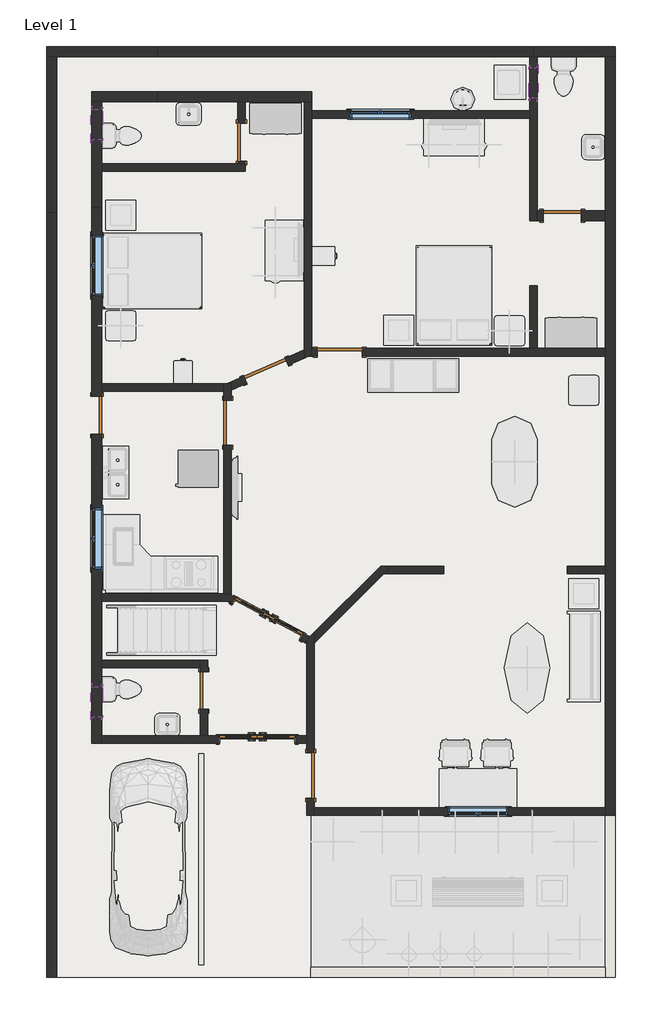
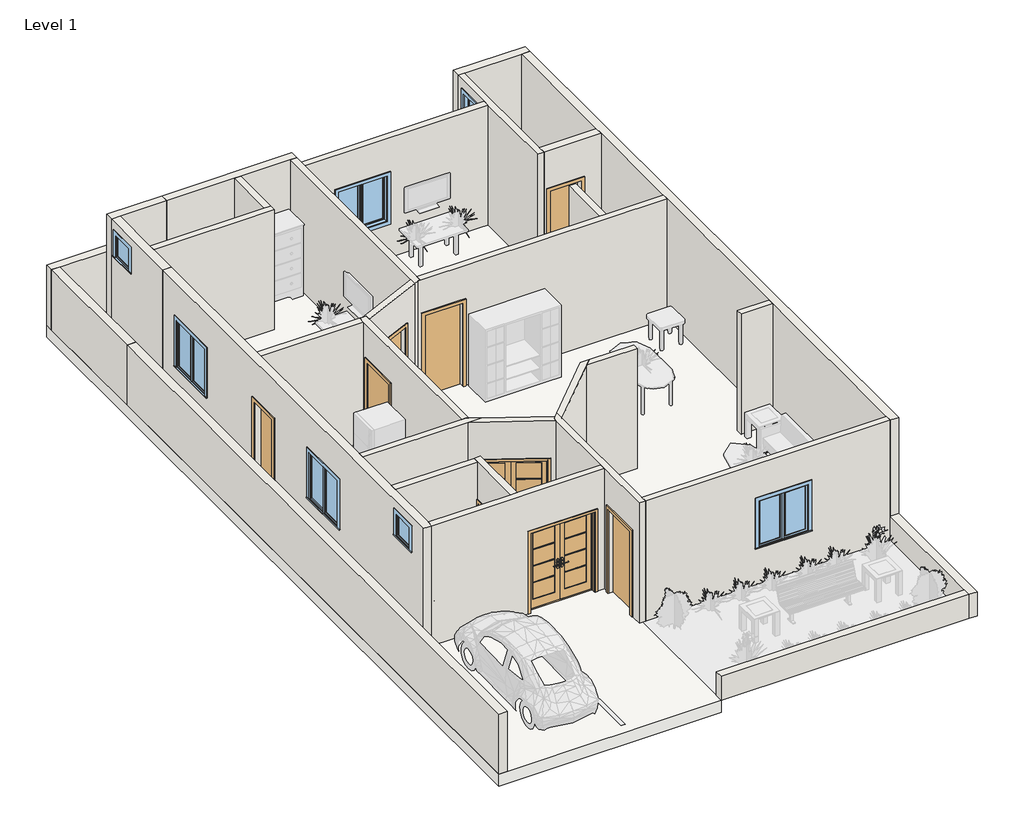
# One storey, part 1 of 2: 33 walls, 10 doors, 7 windows, 1 slab.
"""IFC4 building model written with IfcOpenShell, lengths in millimetres."""

from ifc_helpers import new_model, si_unit, frame, origin, origin_with_axes, place, context, project, spatial, polyline, outline, extrude, faceted_brep, transform, mapped, element, save
from components import door_94998e6c, door_255cab33, door_53b1b562, door_059fdd7e, door_16372e1c, door_686f89d2, window_0862ab64, window_be30da88, window_e41d21a6, window_3d781103

model = new_model("IFC4")

# Units and contexts
model_context = context("Model", 3, world=origin())
ifc_project = project(units=[si_unit("LENGTHUNIT", "METRE", prefix="MILLI")], contexts=[model_context])

# Site, building, storey
site = spatial("IfcSite", under=ifc_project)
building = spatial("IfcBuilding", under=site)
storey = spatial("IfcBuildingStorey", under=building, Name="Level 1", Elevation=0.0)

# Doors
placement = place(None, origin())
door_shape = door_94998e6c(model_context)
element("IfcDoor", 1, ObjectType="Door-Exterior-Double-Full Glass-Wood_Clad : 60\" x 80\"", at=placement, inside=storey, context=model_context, shape_type="MappedRepresentation", body=[
    mapped(door_shape, transform((-8581.0505662, -1172.4507293, 0.0), x_axis=(1.0, 0.0, 0.0), y_axis=(0.0, 1.0, 0.0), z_axis=(0.0, 0.0, 1.0))),
])
element("IfcDoor", 2, ObjectType="Door-Exterior-Double-Full Glass-Wood_Clad : 60\" x 80\"", at=placement, inside=storey, context=model_context, shape_type="MappedRepresentation", body=[
    mapped(door_shape, transform((-8368.5242285, 1268.0386954, 0.0), x_axis=(0.8838359385319597, -0.46779700058821444, 0.0), y_axis=(0.46779700058821444, 0.8838359385319597, 0.0), z_axis=(0.0, 0.0, 1.0))),
])
door_2_shape = door_255cab33(model_context)
element("IfcDoor", 3, ObjectType="Single-Flush : 30\" x 80\"", at=placement, inside=storey, context=model_context, shape_type="MappedRepresentation", body=[
    mapped(door_2_shape, transform((-8898.5505662, 10889.3742707, 0.0), x_axis=(0.0, -1.0, 0.0), y_axis=(1.0, 0.0, 0.0), z_axis=(0.0, 0.0, 1.0))),
])
door_3_shape = door_53b1b562(model_context)
element("IfcDoor", 4, ObjectType="Single-Flush : 30\" x 80\"", at=placement, inside=storey, context=model_context, shape_type="MappedRepresentation", body=[
    mapped(door_3_shape, transform((-11819.5505662, 5375.8598603, 0.0), x_axis=(0.0, 1.0, 0.0), y_axis=(-1.0, 0.0, 0.0), z_axis=(0.0, 0.0, 1.0))),
])
element("IfcDoor", 5, ObjectType="Single-Flush : 30\" x 80\"", at=placement, inside=storey, context=model_context, shape_type="MappedRepresentation", body=[
    mapped(door_3_shape, transform((-2421.5505662, 9403.5067625, 0.0), x_axis=(-1.0, 0.0, 0.0), y_axis=(0.0, -1.0, 0.0), z_axis=(0.0, 0.0, 1.0))),
])
door_4_shape = door_059fdd7e(model_context)
element("IfcDoor", 6, ObjectType="Single-Flush : 30\" x 80\"", at=placement, inside=storey, context=model_context, shape_type="MappedRepresentation", body=[
    mapped(door_4_shape, transform((-9660.5505662, -185.0257293, 0.0), x_axis=(0.0, 1.0, 0.0), y_axis=(-1.0, 0.0, 0.0), z_axis=(0.0, 0.0, 1.0))),
])
door_5_shape = door_16372e1c(model_context)
element("IfcDoor", 7, ObjectType="Single-Flush : 36\" x 84\"", at=placement, inside=storey, context=model_context, shape_type="MappedRepresentation", body=[
    mapped(door_5_shape, transform((-8406.3732014, 6273.0386879, 0.0), x_axis=(0.9158023090349923, 0.40162934500130426, 0.0), y_axis=(-0.40162934500130426, 0.9158023090349923, 0.0), z_axis=(0.0, 0.0, 1.0))),
])
element("IfcDoor", 8, ObjectType="Single-Flush : 36\" x 84\"", at=placement, inside=storey, context=model_context, shape_type="MappedRepresentation", body=[
    mapped(door_5_shape, transform((-9177.9505662, 5223.4598603, 0.0), x_axis=(0.0, 1.0, 0.0), y_axis=(-1.0, 0.0, 0.0), z_axis=(0.0, 0.0, 1.0))),
])
element("IfcDoor", 9, ObjectType="Single-Flush : 36\" x 84\"", at=placement, inside=storey, context=model_context, shape_type="MappedRepresentation", body=[
    mapped(door_5_shape, transform((-7501.5505662, -1899.5257293, 0.0), x_axis=(0.0, -1.0, 0.0), y_axis=(1.0, 0.0, 0.0), z_axis=(0.0, 0.0, 1.0))),
])
door_6_shape = door_686f89d2(model_context)
element("IfcDoor", 10, ObjectType="Single-Flush : 36\" x 84\"", at=placement, inside=storey, context=model_context, shape_type="MappedRepresentation", body=[
    mapped(door_6_shape, transform((-6917.3505662, 6647.5742707, 0.0), x_axis=(-1.0, 0.0, 0.0), y_axis=(0.0, -1.0, 0.0), z_axis=(0.0, 0.0, 1.0))),
])

# Slab
element("IfcSlab", 11, ObjectType="Generic - 12\"", at=placement, inside=storey, context=model_context, shape_type="SweptSolid", body=[
    extrude(outline(polyline([(-1354.7505662, 12819.7742707), (-1354.7505662, -2623.4257293), (-7501.5505662, -2623.4257293), (-7501.5505662, -5823.8257293), (-7501.5505662, -5976.2257293), (-12835.5505662, -5976.2257293), (-12835.5505662, 12819.7742707), (-1354.7505662, 12819.7742707)])), frame((0.0, 0.0, -304.8), z_axis=(0.0, 0.0, 1.0), x_axis=(1.0, 0.0, 0.0)), (0.0, 0.0, 1.0), 304.8),
])

# Walls
element("IfcWall", 12, ObjectType="Generic - 2'", at=placement, inside=storey, context=model_context, shape_type="SweptSolid", body=[
    extrude(outline(polyline([(-7501.5505662, -5773.0257293), (-1557.9505662, -5773.0257293), (-1557.9505662, -5976.2257293), (-7501.5505662, -5976.2257293), (-7501.5505662, -5773.0257293)])), origin_with_axes(), (0.0, 0.0, 1.0), 609.6),
])
element("IfcWall", 13, ObjectType="Generic - 2'", at=placement, inside=storey, context=model_context, shape_type="Brep", body=[
    faceted_brep([(-1557.9505662, -2623.4257293, 0.0), (-1557.9505662, -2699.6257293, 0.0), (-1557.9505662, -5773.0257293, 0.0), (-1557.9505662, -5976.2257293, 0.0), (-1557.9505662, -5976.2257293, 609.6), (-1557.9505662, -5773.0257293, 609.6), (-1557.9505662, -2623.4257293, 609.6), (-1354.7505662, -2623.4257293, 0.0), (-1354.7505662, -2623.4257293, 609.6), (-1354.7505662, -5976.2257293, 609.6), (-1354.7505662, -5976.2257293, 0.0)], [[[0, 1, 2, 3, 4, 5, 6]], [[7, 8, 9, 10]], [[3, 2, 1, 0, 7, 10]], [[6, 5, 4, 9, 8]], [[0, 6, 8, 7]], [[4, 3, 10, 9]]]),
])
element("IfcWall", 14, ObjectType="Generic - 8\"", at=placement, inside=storey, context=model_context, shape_type="Brep", body=[
    faceted_brep([(-1557.9505662, 12616.5742707, 0.0), (-1557.9505662, 9505.1067625, 0.0), (-1557.9505662, 9301.9067625, 0.0), (-1557.9505662, 6723.7742707, 0.0), (-1557.9505662, 6571.3742707, 0.0), (-1557.9505662, 2327.8598603, 0.0), (-1557.9505662, 2175.4598603, 0.0), (-1557.9505662, -2547.2257293, 0.0), (-1557.9505662, -2623.4257293, 0.0), (-1557.9505662, -2623.4257293, 609.6), (-1557.9505662, -2699.6257293, 609.6), (-1557.9505662, -2699.6257293, 3048.0), (-1557.9505662, -2547.2257293, 3048.0), (-1557.9505662, 2175.4598603, 3048.0), (-1557.9505662, 2327.8598603, 3048.0), (-1557.9505662, 6571.3742707, 3048.0), (-1557.9505662, 6723.7742707, 3048.0), (-1557.9505662, 9301.9067625, 3048.0), (-1557.9505662, 9505.1067625, 3048.0), (-1557.9505662, 12616.5742707, 3048.0), (-1354.7505662, 12616.5742707, 0.0), (-1354.7505662, 12616.5742707, 3048.0), (-1354.7505662, -2699.6257293, 3048.0), (-1354.7505662, -2699.6257293, 609.6), (-1354.7505662, -2623.4257293, 609.6), (-1354.7505662, -2623.4257293, 0.0)], [[[0, 1, 2, 3, 4, 5, 6, 7, 8, 9, 10, 11, 12, 13, 14, 15, 16, 17, 18, 19]], [[20, 21, 22, 23, 24, 25]], [[8, 7, 6, 5, 4, 3, 2, 1, 0, 20, 25]], [[0, 19, 21, 20]], [[9, 8, 25, 24]], [[23, 10, 9, 24]], [[11, 10, 23, 22]], [[19, 18, 17, 16, 15, 14, 13, 12, 11, 22, 21]]]),
])
element("IfcWall", 15, ObjectType="Generic - 8\"", at=placement, inside=storey, context=model_context, shape_type="Brep", body=[
    faceted_brep([(-7476.1505662, 11905.3742707, 0.0), (-10600.3505662, 11905.3742707, 0.0), (-10600.3505662, 11905.3742707, 3048.0), (-7476.1505662, 11905.3742707, 3048.0), (-7476.1505662, 11702.1742707, 0.0), (-7476.1505662, 11702.1742707, 3048.0), (-7628.5505662, 11702.1742707, 3048.0), (-8822.3505662, 11702.1742707, 3048.0), (-8974.7505662, 11702.1742707, 3048.0), (-10600.3505662, 11702.1742707, 3048.0), (-10600.3505662, 11702.1742707, 0.0), (-8974.7505662, 11702.1742707, 0.0), (-8822.3505662, 11702.1742707, 0.0), (-7628.5505662, 11702.1742707, 0.0)], [[[0, 1, 2, 3]], [[4, 5, 6, 7, 8, 9, 10, 11, 12, 13]], [[1, 0, 4, 13, 12, 11, 10]], [[2, 1, 10, 9]], [[0, 3, 5, 4]], [[3, 2, 9, 8, 7, 6, 5]]]),
])
element("IfcWall", 16, ObjectType="Generic - 8\"", at=placement, inside=storey, context=model_context, shape_type="Brep", body=[
    faceted_brep([(-11717.9505662, 5756.8598603, 2032.0), (-11717.9505662, 5756.8598603, 0.0), (-11717.9505662, 5858.4598603, 0.0), (-11717.9505662, 6010.8598603, 0.0), (-11717.9505662, 9568.5742707, 0.0), (-11717.9505662, 9568.5742707, 3048.0), (-11717.9505662, 6010.8598603, 3048.0), (-11717.9505662, 5858.4598603, 3048.0), (-11717.9505662, 1769.0598603, 3048.0), (-11717.9505662, 1616.6598603, 3048.0), (-11717.9505662, 424.5742707, 3048.0), (-11717.9505662, 272.1742707, 3048.0), (-11717.9505662, -1099.4257293, 3048.0), (-11717.9505662, -1251.8257293, 3048.0), (-11717.9505662, -1251.8257293, 0.0), (-11717.9505662, -1099.4257293, 0.0), (-11717.9505662, 272.1742707, 0.0), (-11717.9505662, 424.5742707, 0.0), (-11717.9505662, 1616.6598603, 0.0), (-11717.9505662, 1769.0598603, 0.0), (-11717.9505662, 4994.8598603, 0.0), (-11717.9505662, 4994.8598603, 2032.0), (-11717.9505662, 9009.7742707, 2133.6), (-11717.9505662, 9009.7742707, 914.4), (-11717.9505662, 7790.5742707, 914.4), (-11717.9505662, 7790.5742707, 2133.6), (-11717.9505662, 3496.2598603, 2133.6), (-11717.9505662, 3496.2598603, 914.4), (-11717.9505662, 2277.0598603, 914.4), (-11717.9505662, 2277.0598603, 2133.6), (-11717.9505662, -108.8257293, 2768.6), (-11717.9505662, -108.8257293, 2159.0), (-11717.9505662, -718.4257293, 2159.0), (-11717.9505662, -718.4257293, 2768.6), (-11921.1505662, 9568.5742707, 0.0), (-11921.1505662, 5756.8598603, 0.0), (-11921.1505662, 5756.8598603, 2032.0), (-11921.1505662, 4994.8598603, 2032.0), (-11921.1505662, 4994.8598603, 0.0), (-11921.1505662, -1251.8257293, 0.0), (-11921.1505662, -1251.8257293, 3048.0), (-11921.1505662, 9568.5742707, 3048.0), (-11921.1505662, 9009.7742707, 2133.6), (-11921.1505662, 7790.5742707, 2133.6), (-11921.1505662, 7790.5742707, 914.4), (-11921.1505662, 9009.7742707, 914.4), (-11921.1505662, 3496.2598603, 2133.6), (-11921.1505662, 2277.0598603, 2133.6), (-11921.1505662, 2277.0598603, 914.4), (-11921.1505662, 3496.2598603, 914.4), (-11921.1505662, -108.8257293, 2768.6), (-11921.1505662, -718.4257293, 2768.6), (-11921.1505662, -718.4257293, 2159.0), (-11921.1505662, -108.8257293, 2159.0)], [[[0, 1, 2, 3, 4, 5, 6, 7, 8, 9, 10, 11, 12, 13, 14, 15, 16, 17, 18, 19, 20, 21], [22, 23, 24, 25], [26, 27, 28, 29], [30, 31, 32, 33]], [[34, 35, 36, 37, 38, 39, 40, 41], [42, 43, 44, 45], [46, 47, 48, 49], [50, 51, 52, 53]], [[20, 19, 18, 17, 16, 15, 14, 39, 38]], [[4, 3, 2, 1, 35, 34]], [[5, 4, 34, 41]], [[14, 13, 40, 39]], [[36, 35, 1, 0]], [[37, 36, 0, 21]], [[38, 37, 21, 20]], [[23, 22, 42, 45]], [[24, 23, 45, 44]], [[25, 24, 44, 43]], [[22, 25, 43, 42]], [[27, 26, 46, 49]], [[28, 27, 49, 48]], [[29, 28, 48, 47]], [[26, 29, 47, 46]], [[31, 30, 50, 53]], [[32, 31, 53, 52]], [[33, 32, 52, 51]], [[30, 33, 51, 50]], [[13, 12, 11, 10, 9, 8, 7, 6, 5, 41, 40]]]),
])
element("IfcWall", 17, ObjectType="Generic - 8\"", at=placement, inside=storey, context=model_context, shape_type="Brep", body=[
    faceted_brep([(-10600.3505662, 11905.3742707, 0.0), (-11921.1505662, 11905.3742707, 0.0), (-11921.1505662, 11905.3742707, 3048.0), (-10600.3505662, 11905.3742707, 3048.0), (-10600.3505662, 11702.1742707, 0.0), (-10600.3505662, 11702.1742707, 3048.0), (-11717.9505662, 11702.1742707, 3048.0), (-11921.1505662, 11702.1742707, 3048.0), (-11921.1505662, 11702.1742707, 0.0), (-11717.9505662, 11702.1742707, 0.0)], [[[0, 1, 2, 3]], [[4, 5, 6, 7, 8, 9]], [[1, 0, 4, 9, 8]], [[0, 3, 5, 4]], [[2, 1, 8, 7]], [[3, 2, 7, 6, 5]]]),
])
element("IfcWall", 18, ObjectType="Generic - 8\"", at=placement, inside=storey, context=model_context, shape_type="Brep", body=[
    faceted_brep([(-11717.9505662, 9568.5742707, 0.0), (-11717.9505662, 10305.1742707, 0.0), (-11717.9505662, 10457.5742707, 0.0), (-11717.9505662, 11702.1742707, 0.0), (-11717.9505662, 11702.1742707, 3048.0), (-11717.9505662, 10457.5742707, 3048.0), (-11717.9505662, 10305.1742707, 3048.0), (-11717.9505662, 9568.5742707, 3048.0), (-11717.9505662, 11549.7742707, 2768.6), (-11717.9505662, 11549.7742707, 2159.0), (-11717.9505662, 10940.1742707, 2159.0), (-11717.9505662, 10940.1742707, 2768.6), (-11921.1505662, 9568.5742707, 0.0), (-11921.1505662, 9568.5742707, 3048.0), (-11921.1505662, 11702.1742707, 3048.0), (-11921.1505662, 11702.1742707, 0.0), (-11921.1505662, 11549.7742707, 2768.6), (-11921.1505662, 10940.1742707, 2768.6), (-11921.1505662, 10940.1742707, 2159.0), (-11921.1505662, 11549.7742707, 2159.0)], [[[0, 1, 2, 3, 4, 5, 6, 7], [8, 9, 10, 11]], [[12, 13, 14, 15], [16, 17, 18, 19]], [[3, 2, 1, 0, 12, 15]], [[0, 7, 13, 12]], [[4, 3, 15, 14]], [[9, 8, 16, 19]], [[10, 9, 19, 18]], [[11, 10, 18, 17]], [[8, 11, 17, 16]], [[7, 6, 5, 4, 14, 13]]]),
])
element("IfcWall", 19, ObjectType="Generic - 8\"", at=placement, inside=storey, context=model_context, shape_type="SweptSolid", body=[
    extrude(outline(polyline([(0.0, -2929.5505662), (0.0, -2802.5505662), (2032.0, -2802.5505662), (2032.0, -2040.5505662), (0.0, -2040.5505662), (0.0, -1557.9505662), (3048.0, -1557.9505662), (3048.0, -2929.5505662), (0.0, -2929.5505662)])), frame((0.0, 9301.9067625, 0.0), z_axis=(0.0, 1.0, 0.0), x_axis=(0.0, 0.0, 1.0)), (0.0, 0.0, 1.0), 203.2),
])
element("IfcWall", 20, ObjectType="Generic - 8\"", at=placement, inside=storey, context=model_context, shape_type="Brep", body=[
    faceted_brep([(-3005.7505662, 12616.5742707, 0.0), (-2929.5505662, 12616.5742707, 0.0), (-1557.9505662, 12616.5742707, 0.0), (-1354.7505662, 12616.5742707, 0.0), (-1354.7505662, 12616.5742707, 3048.0), (-1557.9505662, 12616.5742707, 3048.0), (-2929.5505662, 12616.5742707, 3048.0), (-3081.9505662, 12616.5742707, 3048.0), (-3081.9505662, 12616.5742707, 1524.0), (-3005.7505662, 12616.5742707, 1524.0), (-3005.7505662, 12819.7742707, 0.0), (-3005.7505662, 12819.7742707, 1524.0), (-3081.9505662, 12819.7742707, 1524.0), (-3081.9505662, 12819.7742707, 3048.0), (-1354.7505662, 12819.7742707, 3048.0), (-1354.7505662, 12819.7742707, 0.0)], [[[0, 1, 2, 3, 4, 5, 6, 7, 8, 9]], [[10, 11, 12, 13, 14, 15]], [[3, 2, 1, 0, 10, 15]], [[4, 3, 15, 14]], [[0, 9, 11, 10]], [[8, 12, 11, 9]], [[8, 7, 13, 12]], [[7, 6, 5, 4, 14, 13]]]),
])
element("IfcWall", 21, ObjectType="INNER 6\"", at=placement, inside=storey, context=model_context, shape_type="Brep", body=[
    faceted_brep([(-7628.5505662, 11702.1742707, 0.0), (-7628.5505662, 6697.3621381, 0.0), (-7628.5505662, 6530.9506774, 0.0), (-7628.5505662, 6530.9506774, 3048.0), (-7628.5505662, 6697.3621381, 3048.0), (-7628.5505662, 11702.1742707, 3048.0), (-7476.1505662, 11702.1742707, 0.0), (-7476.1505662, 11702.1742707, 3048.0), (-7476.1505662, 11524.3742707, 3048.0), (-7476.1505662, 11371.9742707, 3048.0), (-7476.1505662, 6723.7742707, 3048.0), (-7476.1505662, 6597.7864034, 3048.0), (-7476.1505662, 6597.7864034, 0.0), (-7476.1505662, 6723.7742707, 0.0), (-7476.1505662, 11371.9742707, 0.0), (-7476.1505662, 11524.3742707, 0.0), (-7536.3759763, 6571.3742707, 0.0), (-7536.3759763, 6571.3742707, 3048.0)], [[[0, 1, 2, 3, 4, 5]], [[6, 7, 8, 9, 10, 11, 12, 13, 14, 15]], [[2, 1, 0, 6, 15, 14, 13, 12, 16]], [[0, 5, 7, 6]], [[3, 2, 16, 12, 11, 17]], [[5, 4, 3, 17, 11, 10, 9, 8, 7]]]),
])
element("IfcWall", 22, ObjectType="INNER 6\"", at=placement, inside=storey, context=model_context, shape_type="Brep", body=[
    faceted_brep([(-7577.7505662, -2356.7257293, 2133.6), (-7577.7505662, -2356.7257293, 0.0), (-7577.7505662, -2699.6257293, 0.0), (-7577.7505662, -2699.6257293, 3048.0), (-7577.7505662, -1251.8257293, 3048.0), (-7577.7505662, -1099.4257293, 3048.0), (-7577.7505662, 759.6903382, 3048.0), (-7577.7505662, 837.1373442, 3048.0), (-7577.7505662, 837.1373442, 0.0), (-7577.7505662, 759.6903382, 0.0), (-7577.7505662, -1099.4257293, 0.0), (-7577.7505662, -1251.8257293, 0.0), (-7577.7505662, -1442.3257293, 0.0), (-7577.7505662, -1442.3257293, 2133.6), (-7425.3505662, -2699.6257293, 0.0), (-7425.3505662, -2547.2257293, 0.0), (-7425.3505662, -2356.7257293, 0.0), (-7425.3505662, -2356.7257293, 2133.6), (-7425.3505662, -1442.3257293, 2133.6), (-7425.3505662, -1442.3257293, 0.0), (-7425.3505662, 774.0111973, 0.0), (-7425.3505662, 989.5373442, 0.0), (-7425.3505662, 989.5373442, 3048.0), (-7425.3505662, 774.0111973, 3048.0), (-7425.3505662, -2547.2257293, 3048.0), (-7425.3505662, -2699.6257293, 3048.0), (-7515.6408392, 899.2470712, 0.0), (-7515.6408392, 899.2470712, 3048.0)], [[[0, 1, 2, 3, 4, 5, 6, 7, 8, 9, 10, 11, 12, 13]], [[14, 15, 16, 17, 18, 19, 20, 21, 22, 23, 24, 25]], [[2, 1, 16, 15, 14]], [[12, 11, 10, 9, 8, 26, 21, 20, 19]], [[3, 2, 14, 25]], [[8, 7, 27, 22, 21, 26]], [[17, 16, 1, 0]], [[18, 17, 0, 13]], [[19, 18, 13, 12]], [[7, 6, 5, 4, 3, 25, 24, 23, 22, 27]]]),
])
element("IfcWall", 23, ObjectType="INNER 6\"", at=placement, inside=storey, context=model_context, shape_type="Brep", body=[
    faceted_brep([(-7425.3505662, -2699.6257293, 0.0), (-1557.9505662, -2699.6257293, 0.0), (-1557.9505662, -2699.6257293, 609.6), (-1557.9505662, -2699.6257293, 3048.0), (-7425.3505662, -2699.6257293, 3048.0), (-4732.9505662, -2699.6257293, 2133.6), (-3513.7505662, -2699.6257293, 2133.6), (-3513.7505662, -2699.6257293, 914.4), (-4732.9505662, -2699.6257293, 914.4), (-7425.3505662, -2547.2257293, 0.0), (-7425.3505662, -2547.2257293, 3048.0), (-1557.9505662, -2547.2257293, 3048.0), (-1557.9505662, -2547.2257293, 0.0), (-4732.9505662, -2547.2257293, 2133.6), (-4732.9505662, -2547.2257293, 914.4), (-3513.7505662, -2547.2257293, 914.4), (-3513.7505662, -2547.2257293, 2133.6), (-1557.9505662, -2623.4257293, 0.0)], [[[0, 1, 2, 3, 4], [5, 6, 7, 8]], [[9, 10, 11, 12], [13, 14, 15, 16]], [[1, 0, 9, 12, 17]], [[0, 4, 10, 9]], [[14, 13, 5, 8]], [[15, 14, 8, 7]], [[16, 15, 7, 6]], [[13, 16, 6, 5]], [[1, 17, 12, 11, 3, 2]], [[4, 3, 11, 10]]]),
])
element("IfcWall", 24, ObjectType="INNER 6\"", at=placement, inside=storey, context=model_context, shape_type="Brep", body=[
    faceted_brep([(-7577.7505662, -1099.4257293, 3048.0), (-7577.7505662, -1099.4257293, 0.0), (-7793.6505662, -1099.4257293, 0.0), (-7793.6505662, -1099.4257293, 2057.4), (-9368.4505662, -1099.4257293, 2057.4), (-9368.4505662, -1099.4257293, 0.0), (-9584.3505662, -1099.4257293, 0.0), (-9736.7505662, -1099.4257293, 0.0), (-11717.9505662, -1099.4257293, 0.0), (-11717.9505662, -1099.4257293, 3048.0), (-9736.7505662, -1099.4257293, 3048.0), (-9584.3505662, -1099.4257293, 3048.0), (-7577.7505662, -1251.8257293, 0.0), (-7577.7505662, -1251.8257293, 3048.0), (-11717.9505662, -1251.8257293, 3048.0), (-11717.9505662, -1251.8257293, 0.0), (-9368.4505662, -1251.8257293, 0.0), (-9368.4505662, -1251.8257293, 2057.4), (-7793.6505662, -1251.8257293, 2057.4), (-7793.6505662, -1251.8257293, 0.0)], [[[0, 1, 2, 3, 4, 5, 6, 7, 8, 9, 10, 11]], [[12, 13, 14, 15, 16, 17, 18, 19]], [[1, 12, 19, 2]], [[15, 8, 7, 6, 5, 16]], [[1, 0, 13, 12]], [[9, 8, 15, 14]], [[18, 3, 2, 19]], [[3, 18, 17, 4]], [[4, 17, 16, 5]], [[0, 11, 10, 9, 14, 13]]]),
])
element("IfcWall", 25, ObjectType="INNER 6\"", at=placement, inside=storey, context=model_context, shape_type="Brep", body=[
    faceted_brep([(-7425.3505662, 774.0111973, 0.0), (-6023.9019032, 2175.4598603, 0.0), (-5871.5019032, 2327.8598603, 0.0), (-5871.5019032, 2327.8598603, 3048.0), (-6023.9019032, 2175.4598603, 3048.0), (-7425.3505662, 774.0111973, 3048.0), (-7425.3505662, 989.5373442, 0.0), (-7425.3505662, 989.5373442, 3048.0), (-6087.0280501, 2327.8598603, 3048.0), (-6087.0280501, 2327.8598603, 0.0)], [[[0, 1, 2, 3, 4, 5]], [[6, 7, 8, 9]], [[2, 1, 0, 6, 9]], [[0, 5, 7, 6]], [[3, 2, 9, 8]], [[5, 4, 3, 8, 7]]]),
])
element("IfcWall", 26, ObjectType="INNER 6\"", at=placement, inside=storey, context=model_context, shape_type="SweptSolid", body=[
    extrude(outline(polyline([(-4810.8649766, 2175.4598603), (-6023.9019032, 2175.4598603), (-5871.5019032, 2327.8598603), (-4810.8649766, 2327.8598603), (-4810.8649766, 2175.4598603)])), origin_with_axes(), (0.0, 0.0, 1.0), 3048.0),
])
element("IfcWall", 27, ObjectType="INNER 6\"", at=placement, inside=storey, context=model_context, shape_type="Brep", body=[
    faceted_brep([(-9584.3505662, 195.9742707, 2032.0), (-9584.3505662, 195.9742707, 0.0), (-9584.3505662, 424.5742707, 0.0), (-9584.3505662, 424.5742707, 3048.0), (-9584.3505662, -1099.4257293, 3048.0), (-9584.3505662, -1099.4257293, 0.0), (-9584.3505662, -566.0257293, 0.0), (-9584.3505662, -566.0257293, 2032.0), (-9736.7505662, 424.5742707, 0.0), (-9736.7505662, 272.1742707, 0.0), (-9736.7505662, 195.9742707, 0.0), (-9736.7505662, 195.9742707, 2032.0), (-9736.7505662, -566.0257293, 2032.0), (-9736.7505662, -566.0257293, 0.0), (-9736.7505662, -1099.4257293, 0.0), (-9736.7505662, -1099.4257293, 3048.0), (-9736.7505662, 272.1742707, 3048.0), (-9736.7505662, 424.5742707, 3048.0)], [[[0, 1, 2, 3, 4, 5, 6, 7]], [[8, 9, 10, 11, 12, 13, 14, 15, 16, 17]], [[6, 5, 14, 13]], [[2, 1, 10, 9, 8]], [[5, 4, 15, 14]], [[3, 2, 8, 17]], [[11, 10, 1, 0]], [[12, 11, 0, 7]], [[13, 12, 7, 6]], [[4, 3, 17, 16, 15]]]),
])
element("IfcWall", 28, ObjectType="INNER 6\"", at=placement, inside=storey, context=model_context, shape_type="SweptSolid", body=[
    extrude(outline(polyline([(-11717.9505662, 424.5742707), (-9736.7505662, 424.5742707), (-9736.7505662, 272.1742707), (-11717.9505662, 272.1742707), (-11717.9505662, 424.5742707)])), origin_with_axes(), (0.0, 0.0, 1.0), 3048.0),
])
element("IfcWall", 29, ObjectType="INNER 6\"", at=placement, inside=storey, context=model_context, shape_type="Brep", body=[
    faceted_brep([(-11717.9505662, 1616.6598603, 3048.0), (-11717.9505662, 1616.6598603, 0.0), (-9196.8726659, 1616.6598603, 0.0), (-9074.8952161, 1616.6598603, 0.0), (-9074.8952161, 1616.6598603, 2057.4), (-8871.0903291, 1616.6598603, 2057.4), (-8871.0903291, 1616.6598603, 3048.0), (-9196.8726659, 1616.6598603, 3048.0), (-9159.0284665, 1769.0598603, 0.0), (-9254.1505662, 1769.0598603, 0.0), (-11717.9505662, 1769.0598603, 0.0), (-11717.9505662, 1769.0598603, 3048.0), (-9254.1505662, 1769.0598603, 3048.0), (-9159.0284665, 1769.0598603, 3048.0), (-9101.7505662, 1738.7437928, 0.0), (-9030.2957705, 1700.9241731, 0.0), (-9101.7505662, 1738.7437928, 3048.0), (-9030.2957705, 1700.9241731, 2057.4)], [[[0, 1, 2, 3, 4, 5, 6, 7]], [[8, 9, 10, 11, 12, 13]], [[10, 9, 8, 14, 15, 3, 2, 1]], [[1, 0, 11, 10]], [[8, 13, 16, 6, 5, 17, 15, 14]], [[4, 17, 5]], [[17, 4, 3, 15]], [[0, 7, 6, 16, 13, 12, 11]]]),
])
element("IfcWall", 30, ObjectType="INNER 6\"", at=placement, inside=storey, context=model_context, shape_type="Brep", body=[
    faceted_brep([(-7577.7505662, 759.6903382, 0.0), (-7577.7505662, 759.6903382, 3048.0), (-9196.8726659, 1616.6598603, 3048.0), (-9196.8726659, 1616.6598603, 0.0), (-9101.5880334, 1566.2275761, 0.0), (-9101.5880334, 1566.2275761, 2057.4), (-7709.7231974, 829.5408595, 2057.4), (-7709.7231974, 829.5408595, 0.0), (-7515.6408392, 899.2470712, 3048.0), (-7515.6408392, 899.2470712, 0.0), (-7638.4309345, 964.2374566, 0.0), (-7638.4309345, 964.2374566, 2057.4), (-8871.0903291, 1616.6598603, 2057.4), (-8871.0903291, 1616.6598603, 3048.0), (-7577.7505662, 837.1373442, 0.0), (-9074.8952161, 1616.6598603, 0.0), (-7577.7505662, 837.1373442, 3048.0), (-9074.8952161, 1616.6598603, 2057.4)], [[[0, 1, 2, 3, 4, 5, 6, 7]], [[8, 9, 10, 11, 12, 13]], [[9, 14, 0, 7, 10]], [[4, 3, 15]], [[1, 0, 14, 16]], [[9, 8, 16, 14]], [[3, 2, 13, 12, 17, 15]], [[6, 11, 10, 7]], [[11, 6, 5, 17, 12]], [[17, 5, 4, 15]], [[2, 1, 16, 8, 13]]]),
])
element("IfcWall", 31, ObjectType="INNER 6\"", at=placement, inside=storey, context=model_context, shape_type="Brep", body=[
    faceted_brep([(-9101.7505662, 5680.6598603, 2133.6), (-9101.7505662, 5680.6598603, 0.0), (-9101.7505662, 5884.8719929, 0.0), (-9101.7505662, 6010.8598603, 0.0), (-9101.7505662, 6010.8598603, 3048.0), (-9101.7505662, 5884.8719929, 3048.0), (-9101.7505662, 1738.7437928, 3048.0), (-9101.7505662, 1738.7437928, 0.0), (-9101.7505662, 4766.2598603, 0.0), (-9101.7505662, 4766.2598603, 2133.6), (-9254.1505662, 6010.8598603, 0.0), (-9254.1505662, 5858.4598603, 0.0), (-9254.1505662, 5680.6598603, 0.0), (-9254.1505662, 5680.6598603, 2133.6), (-9254.1505662, 4766.2598603, 2133.6), (-9254.1505662, 4766.2598603, 0.0), (-9254.1505662, 1769.0598603, 0.0), (-9254.1505662, 1769.0598603, 3048.0), (-9254.1505662, 5858.4598603, 3048.0), (-9254.1505662, 6010.8598603, 3048.0), (-9159.0284665, 1769.0598603, 0.0), (-9193.925156, 6010.8598603, 0.0), (-9159.0284665, 1769.0598603, 3048.0), (-9193.925156, 6010.8598603, 3048.0)], [[[0, 1, 2, 3, 4, 5, 6, 7, 8, 9]], [[10, 11, 12, 13, 14, 15, 16, 17, 18, 19]], [[8, 7, 20, 16, 15]], [[3, 2, 1, 12, 11, 10, 21]], [[7, 6, 22, 20]], [[22, 17, 16, 20]], [[4, 3, 21, 10, 19, 23]], [[13, 12, 1, 0]], [[14, 13, 0, 9]], [[15, 14, 9, 8]], [[6, 5, 4, 23, 19, 18, 17, 22]]]),
])
element("IfcWall", 32, ObjectType="INNER 6\"", at=placement, inside=storey, context=model_context, shape_type="SweptSolid", body=[
    extrude(outline(polyline([(-11717.9505662, 6010.8598603), (-9254.1505662, 6010.8598603), (-9254.1505662, 5858.4598603), (-11717.9505662, 5858.4598603), (-11717.9505662, 6010.8598603)])), origin_with_axes(), (0.0, 0.0, 1.0), 3048.0),
])
element("IfcWall", 33, ObjectType="INNER 6\"", at=placement, inside=storey, context=model_context, shape_type="Brep", body=[
    faceted_brep([(-7957.0642296, 6386.8794885, 2133.6), (-7957.0642296, 6386.8794885, 0.0), (-7628.5505662, 6530.9506774, 0.0), (-7628.5505662, 6530.9506774, 3048.0), (-9101.7505662, 5884.8719929, 3048.0), (-9101.7505662, 5884.8719929, 0.0), (-8794.473861, 6019.6296154, 0.0), (-8794.473861, 6019.6296154, 2133.6), (-7628.5505662, 6697.3621381, 0.0), (-8018.2725418, 6526.4477604, 0.0), (-8018.2725418, 6526.4477604, 2133.6), (-8855.6821732, 6159.1978873, 2133.6), (-8855.6821732, 6159.1978873, 0.0), (-9193.925156, 6010.8598603, 0.0), (-9193.925156, 6010.8598603, 3048.0), (-7628.5505662, 6697.3621381, 3048.0), (-9101.7505662, 6010.8598603, 0.0), (-9101.7505662, 6010.8598603, 3048.0)], [[[0, 1, 2, 3, 4, 5, 6, 7]], [[8, 9, 10, 11, 12, 13, 14, 15]], [[6, 5, 16, 13, 12]], [[2, 1, 9, 8]], [[3, 2, 8, 15]], [[5, 4, 17, 16]], [[17, 14, 13, 16]], [[10, 9, 1, 0]], [[11, 10, 0, 7]], [[12, 11, 7, 6]], [[4, 3, 15, 14, 17]]]),
])
element("IfcWall", 34, ObjectType="INNER 6\"", at=placement, inside=storey, context=model_context, shape_type="SweptSolid", body=[
    extrude(outline(polyline([(0.0, -7476.1505662), (0.0, -3081.9505662), (3048.0, -3081.9505662), (3048.0, -7476.1505662), (0.0, -7476.1505662)]), holes=[polyline([(2133.6, -5482.2505662), (914.4, -5482.2505662), (914.4, -6701.4505662), (2133.6, -6701.4505662), (2133.6, -5482.2505662)])]), frame((0.0, 11371.9742707, 0.0), z_axis=(0.0, 1.0, 0.0), x_axis=(0.0, 0.0, 1.0)), (0.0, 0.0, 1.0), 152.4),
])
element("IfcWall", 35, ObjectType="INNER 6\"", at=placement, inside=storey, context=model_context, shape_type="Brep", body=[
    faceted_brep([(-7536.3759763, 6571.3742707, 0.0), (-7374.5505662, 6571.3742707, 0.0), (-7374.5505662, 6571.3742707, 2133.6), (-6460.1505662, 6571.3742707, 2133.6), (-6460.1505662, 6571.3742707, 0.0), (-1557.9505662, 6571.3742707, 0.0), (-1557.9505662, 6571.3742707, 3048.0), (-7536.3759763, 6571.3742707, 3048.0), (-7374.5505662, 6723.7742707, 2133.6), (-7374.5505662, 6723.7742707, 0.0), (-7476.1505662, 6723.7742707, 0.0), (-7476.1505662, 6723.7742707, 3048.0), (-3081.9505662, 6723.7742707, 3048.0), (-2929.5505662, 6723.7742707, 3048.0), (-1557.9505662, 6723.7742707, 3048.0), (-1557.9505662, 6723.7742707, 0.0), (-2929.5505662, 6723.7742707, 0.0), (-3081.9505662, 6723.7742707, 0.0), (-6460.1505662, 6723.7742707, 0.0), (-6460.1505662, 6723.7742707, 2133.6), (-7476.1505662, 6597.7864034, 0.0), (-7476.1505662, 6597.7864034, 3048.0)], [[[0, 1, 2, 3, 4, 5, 6, 7]], [[8, 9, 10, 11, 12, 13, 14, 15, 16, 17, 18, 19]], [[10, 9, 1, 0, 20]], [[18, 17, 16, 15, 5, 4]], [[0, 7, 21, 20]], [[21, 11, 10, 20]], [[6, 5, 15, 14]], [[2, 1, 9, 8]], [[3, 2, 8, 19]], [[4, 3, 19, 18]], [[7, 6, 14, 13, 12, 11, 21]]]),
])
element("IfcWall", 36, ObjectType="INNER 6\"", at=placement, inside=storey, context=model_context, shape_type="Brep", body=[
    faceted_brep([(-11717.9505662, 10305.1742707, 0.0), (-8822.3505662, 10305.1742707, 0.0), (-8822.3505662, 10305.1742707, 3048.0), (-11717.9505662, 10305.1742707, 3048.0), (-11717.9505662, 10457.5742707, 0.0), (-11717.9505662, 10457.5742707, 3048.0), (-8974.7505662, 10457.5742707, 3048.0), (-8822.3505662, 10457.5742707, 3048.0), (-8822.3505662, 10457.5742707, 0.0), (-8974.7505662, 10457.5742707, 0.0)], [[[0, 1, 2, 3]], [[4, 5, 6, 7, 8, 9]], [[1, 0, 4, 9, 8]], [[0, 3, 5, 4]], [[2, 1, 8, 7]], [[3, 2, 7, 6, 5]]]),
])
element("IfcWall", 37, ObjectType="INNER 6\"", at=placement, inside=storey, context=model_context, shape_type="SweptSolid", body=[
    extrude(outline(polyline([(10508.3742707, 2032.0), (10508.3742707, 0.0), (10457.5742707, 0.0), (10457.5742707, 3048.0), (11702.1742707, 3048.0), (11702.1742707, 0.0), (11270.3742707, 0.0), (11270.3742707, 2032.0), (10508.3742707, 2032.0)])), frame((-8974.7505662, 0.0, 0.0), z_axis=(1.0, 0.0, 0.0), x_axis=(0.0, 1.0, 0.0)), (0.0, 0.0, 1.0), 152.4),
])
element("IfcWall", 38, ObjectType="INNER 6\"", at=placement, inside=storey, context=model_context, shape_type="SweptSolid", body=[
    extrude(outline(polyline([(-1557.9505662, 2175.4598603), (-2319.9505662, 2175.4598603), (-2319.9505662, 2327.8598603), (-1557.9505662, 2327.8598603), (-1557.9505662, 2175.4598603)])), origin_with_axes(), (0.0, 0.0, 1.0), 3048.0),
])
element("IfcWall", 39, ObjectType="INNER 6\"", at=placement, inside=storey, context=model_context, shape_type="Brep", body=[
    faceted_brep([(-2929.5505662, 9301.9067625, 0.0), (-2929.5505662, 9505.1067625, 0.0), (-2929.5505662, 12616.5742707, 0.0), (-2929.5505662, 12616.5742707, 3048.0), (-2929.5505662, 9505.1067625, 3048.0), (-2929.5505662, 9301.9067625, 3048.0), (-2929.5505662, 11778.3742707, 2768.6), (-2929.5505662, 12387.9742707, 2768.6), (-2929.5505662, 12387.9742707, 2159.0), (-2929.5505662, 11778.3742707, 2159.0), (-3081.9505662, 9301.9067625, 0.0), (-3081.9505662, 9301.9067625, 3048.0), (-3081.9505662, 11371.9742707, 3048.0), (-3081.9505662, 11524.3742707, 3048.0), (-3081.9505662, 12616.5742707, 3048.0), (-3081.9505662, 12616.5742707, 1524.0), (-3081.9505662, 12616.5742707, 0.0), (-3081.9505662, 11524.3742707, 0.0), (-3081.9505662, 11371.9742707, 0.0), (-3081.9505662, 11778.3742707, 2768.6), (-3081.9505662, 11778.3742707, 2159.0), (-3081.9505662, 12387.9742707, 2159.0), (-3081.9505662, 12387.9742707, 2768.6), (-3005.7505662, 12616.5742707, 0.0)], [[[0, 1, 2, 3, 4, 5], [6, 7, 8, 9]], [[10, 11, 12, 13, 14, 15, 16, 17, 18], [19, 20, 21, 22]], [[2, 1, 0, 10, 18, 17, 16, 23]], [[0, 5, 11, 10]], [[20, 19, 6, 9]], [[21, 20, 9, 8]], [[22, 21, 8, 7]], [[19, 22, 7, 6]], [[2, 23, 16, 15, 14, 3]], [[5, 4, 3, 14, 13, 12, 11]]]),
])
element("IfcWall", 40, ObjectType="INNER 6\"", at=placement, inside=storey, context=model_context, shape_type="SweptSolid", body=[
    extrude(outline(polyline([(-3081.9505662, 6723.7742707), (-3081.9505662, 7993.7742707), (-2929.5505662, 7993.7742707), (-2929.5505662, 6723.7742707), (-3081.9505662, 6723.7742707)])), origin_with_axes(), (0.0, 0.0, 1.0), 3048.0),
])
element("IfcWall", 41, ObjectType="OUTER 5'", at=placement, inside=storey, context=model_context, shape_type="Brep", body=[
    faceted_brep([(-12835.5505662, 12616.5742707, 0.0), (-12632.3505662, 12616.5742707, 0.0), (-10600.3505662, 12616.5742707, 0.0), (-10600.3505662, 12616.5742707, 1524.0), (-12632.3505662, 12616.5742707, 1524.0), (-12835.5505662, 12616.5742707, 1524.0), (-12835.5505662, 12819.7742707, 0.0), (-12835.5505662, 12819.7742707, 1524.0), (-10600.3505662, 12819.7742707, 1524.0), (-10600.3505662, 12819.7742707, 0.0)], [[[0, 1, 2, 3, 4, 5]], [[6, 7, 8, 9]], [[2, 1, 0, 6, 9]], [[3, 2, 9, 8]], [[5, 4, 3, 8, 7]], [[0, 5, 7, 6]]]),
])
element("IfcWall", 42, ObjectType="OUTER 5'", at=placement, inside=storey, context=model_context, shape_type="SweptSolid", body=[
    extrude(outline(polyline([(-12632.3505662, 9466.9742707), (-12632.3505662, -5976.2257293), (-12835.5505662, -5976.2257293), (-12835.5505662, 9466.9742707), (-12632.3505662, 9466.9742707)])), origin_with_axes(), (0.0, 0.0, 1.0), 1524.0),
])
element("IfcWall", 43, ObjectType="OUTER 5'", at=placement, inside=storey, context=model_context, shape_type="Brep", body=[
    faceted_brep([(-10600.3505662, 12616.5742707, 0.0), (-3081.9505662, 12616.5742707, 0.0), (-3005.7505662, 12616.5742707, 0.0), (-3005.7505662, 12616.5742707, 1524.0), (-10600.3505662, 12616.5742707, 1524.0), (-10600.3505662, 12819.7742707, 0.0), (-10600.3505662, 12819.7742707, 1524.0), (-3005.7505662, 12819.7742707, 1524.0), (-3005.7505662, 12819.7742707, 0.0)], [[[0, 1, 2, 3, 4]], [[5, 6, 7, 8]], [[2, 1, 0, 5, 8]], [[3, 2, 8, 7]], [[4, 3, 7, 6]], [[0, 4, 6, 5]]]),
])
element("IfcWall", 44, ObjectType="OUTER 5'", at=placement, inside=storey, context=model_context, shape_type="SweptSolid", body=[
    extrude(outline(polyline([(-12632.3505662, 12616.5742707), (-12632.3505662, 9466.9742707), (-12835.5505662, 9466.9742707), (-12835.5505662, 12616.5742707), (-12632.3505662, 12616.5742707)])), origin_with_axes(), (0.0, 0.0, 1.0), 1524.0),
])

# Windows
window_shape = window_0862ab64(model_context)
element("IfcWindow", 45, ObjectType="Casement Dbl with Trim : 48\" x 48\"", at=placement, inside=storey, context=model_context, shape_type="MappedRepresentation", body=[
    mapped(window_shape, transform((-11800.5005662, 8400.1742707, 0.0), x_axis=(0.0, 1.0, 0.0), y_axis=(-1.0, 0.0, 0.0), z_axis=(0.0, 0.0, 1.0))),
])
element("IfcWindow", 46, ObjectType="Casement Dbl with Trim : 48\" x 48\"", at=placement, inside=storey, context=model_context, shape_type="MappedRepresentation", body=[
    mapped(window_shape, transform((-11800.5005662, 2886.6598603, 0.0), x_axis=(0.0, 1.0, 0.0), y_axis=(-1.0, 0.0, 0.0), z_axis=(0.0, 0.0, 1.0))),
])
window_2_shape = window_be30da88(model_context)
element("IfcWindow", 47, ObjectType="Casement Dbl with Trim : 48\" x 48\"", at=placement, inside=storey, context=model_context, shape_type="MappedRepresentation", body=[
    mapped(window_2_shape, transform((-4123.3505662, -2604.3757293, 0.0), x_axis=(-1.0, 0.0, 0.0), y_axis=(0.0, -1.0, 0.0), z_axis=(0.0, 0.0, 1.0))),
])
element("IfcWindow", 48, ObjectType="Casement Dbl with Trim : 48\" x 48\"", at=placement, inside=storey, context=model_context, shape_type="MappedRepresentation", body=[
    mapped(window_2_shape, transform((-6091.8505662, 11429.1242707, 0.0), x_axis=(1.0, 0.0, 0.0), y_axis=(0.0, 1.0, 0.0), z_axis=(0.0, 0.0, 1.0))),
])
window_3_shape = window_e41d21a6(model_context)
element("IfcWindow", 49, ObjectType="Transom with Trim : 24\" x 24\"", at=placement, inside=storey, context=model_context, shape_type="MappedRepresentation", body=[
    mapped(window_3_shape, transform((-11819.5505662, -375.5257293, 0.0), x_axis=(0.0, 1.0, 0.0), y_axis=(-1.0, 0.0, 0.0), z_axis=(0.0, 0.0, 1.0))),
])
element("IfcWindow", 50, ObjectType="Transom with Trim : 24\" x 24\"", at=placement, inside=storey, context=model_context, shape_type="MappedRepresentation", body=[
    mapped(window_3_shape, transform((-11819.5505662, 11283.0742707, 0.0), x_axis=(0.0, 1.0, 0.0), y_axis=(-1.0, 0.0, 0.0), z_axis=(0.0, 0.0, 1.0))),
])
window_4_shape = window_3d781103(model_context)
element("IfcWindow", 51, ObjectType="Transom with Trim : 24\" x 24\"", at=placement, inside=storey, context=model_context, shape_type="MappedRepresentation", body=[
    mapped(window_4_shape, transform((-3005.7505662, 12045.0742707, 0.0), x_axis=(0.0, -1.0, 0.0), y_axis=(1.0, 0.0, 0.0), z_axis=(0.0, 0.0, 1.0))),
])

save(model, "model.ifc")

# Revit data of these elements
# Type "Door-Exterior-Double-Full Glass-Wood_Clad : 60\" x 80\""
#   Type Mark = "8"
#   Assembly Code = "B2030100"
#   Analytic Construction = "French door, wood frame with double glass"
#   Top Rail = 0' - 4 11/16"
#   Threshold Offset [instance default] = 0' - 0 1/2"
#   Thickness = 0' - 1 3/8"
#   Thermal Resistance (R) = 1.9158 (h·ft²·°F)/BTU
#   Swing Angle [instance default] = 90.00°
#   Stiles = 0' - 4 3/4"
#   Rough Width = 5' - 2"
#   Rough Height = 6' - 9"
#   Panel Width = 2' - 6"
#   Door Offset [instance default] = 0' - 0"
#   Height = 6' - 8"
#   Width = 5' - 0"
#   Heat Transfer Coefficient (U) = 0.5220 BTU/(h·ft²·°F)
#   Bottom Rail = 0' - 9 1/8"
#   Exterior Trim [instance default] = yes
#   Threshold [instance default] = yes
#   Show Grill [instance default] = yes
#   Function = 1
#   Trim Material = Cherry
#   Threshold Material = Cherry
#   Panel Material = Cherry
#   Glazing = Glass
#   Frame Material = Cherry
#   Door Handle Material = Aluminum
#   Visual Light Transmittance = 0
#   Solar Heat Gain Coefficient = 0
#   Wall Closure = (empty or 0)
#   Construction Type = (empty or 0)
# Type "Single-Flush : 30\" x 80\""
#   Type Mark = "5"
#   Construction Type Id = "MDOOR"
#   Assembly Code = "C1020"
#   Analytic Construction = "Metal"
#   Thickness = 0' - 2"
#   Heat Transfer Coefficient (U) = 0.651978 BTU/(h·ft²·°F)
#   Height = 6' - 8"
#   Trim Projection Ext = 0' - 1"
#   Trim Projection Int = 0' - 1"
#   Trim Width = 0' - 3"
#   Width = 2' - 6"
#   Define Thermal Properties by = 1
#   Door Material = Door - Panel
#   Frame Material = Door - Frame
#   Visual Light Transmittance = 0
#   Solar Heat Gain Coefficient = 0
#   Function = (empty or 0)
#   Wall Closure = (empty or 0)
# Type "Single-Flush : 36\" x 84\""
#   Type Mark = "1"
#   Construction Type Id = "MDOOR"
#   Assembly Code = "C1020"
#   Analytic Construction = "Metal"
#   Thickness = 0' - 2"
#   Heat Transfer Coefficient (U) = 0.651978 BTU/(h·ft²·°F)
#   Height = 7' - 0"
#   Trim Projection Ext = 0' - 1"
#   Trim Projection Int = 0' - 1"
#   Trim Width = 0' - 3"
#   Width = 3' - 0"
#   Define Thermal Properties by = 1
#   Door Material = Door - Panel
#   Frame Material = Door - Frame
#   Visual Light Transmittance = 0
#   Solar Heat Gain Coefficient = 0
#   Function = (empty or 0)
#   Wall Closure = (empty or 0)
# Type "Generic - 12\""
#   Assembly Code = "B1010"
#   Function = 0
#   Layers, outside or top first: 1' - 0" no material (function 1)
# Type "Generic - 2'"
#   Assembly Code = "B2010"
#   Layers, outside or top first: 0' - 8" "Birch" (function 1)
# Type "Generic - 8\""
#   Assembly Code = "B2010"
#   Layers, outside or top first: 0' - 8" "Brick, Common" (function 1)
# Type "INNER 6\""
#   Assembly Code = "B2010"
#   Layers, outside or top first: 0' - 6" "Brick, Common" (function 1)
# Type "OUTER 5'"
#   Assembly Code = "B2010"
#   Layers, outside or top first: 0' - 8" "Birch" (function 1)
# Type "Casement Dbl with Trim : 48\" x 48\""
#   Type Mark = "10"
#   Construction Type Id = "GSP4R"
#   Assembly Code = "B2020100"
#   Analytic Construction = "1/8 in Pilkington single glazing"
#   Visual Light Transmittance = 0.9
#   Solar Heat Gain Coefficient = 0.78
#   Heat Transfer Coefficient (U) = 0.6496 BTU/(h·ft²·°F)
#   Height = 4' - 0"
#   Default Sill Height = 3' - 0"
#   Trim Projection - Ext. = 0' - 0 1/2"
#   Trim Projection - Int. = 0' - 0 3/4"
#   Trim Width - Exterior = 0' - 3 1/2"
#   Trim Width - Interior = 0' - 3 1/2"
#   Width = 4' - 0"
#   Window Inset = 0' - 0 3/4"
#   Define Thermal Properties by = 1
#   Glass Pane Material = Glass
#   Sash Material = Sash
#   Trim Exterior Material = Trim
#   Trim Interior Material = Trim
#   Wall Closure = (empty or 0)
# Type "Transom with Trim : 24\" x 24\""
#   Type Mark = "13"
#   Construction Type Id = "GSP4R"
#   Assembly Code = "B2020100"
#   Analytic Construction = "1/8 in Pilkington single glazing"
#   Visual Light Transmittance = 0.9
#   Solar Heat Gain Coefficient = 0.78
#   Heat Transfer Coefficient (U) = 0.6496 BTU/(h·ft²·°F)
#   Height = 2' - 0"
#   Default Sill Height = 7' - 1"
#   Trim Projection - Ext. = 0' - 0 1/2"
#   Trim Projection - Int. = 0' - 0 3/4"
#   Trim Width - Exterior = 0' - 3 1/2"
#   Trim Width - Interior = 0' - 3 1/2"
#   Width = 2' - 0"
#   Window Inset = 0' - 0 3/4"
#   Define Thermal Properties by = 1
#   Glass Pane Material = Glass
#   Sash Material = Sash
#   Trim Exterior Material = Trim
#   Trim Interior Material = Trim
#   Wall Closure = (empty or 0)
# Elements 1, 2 (IfcDoor, "Door-Exterior-Double-Full Glass-Wood_Clad : 60\" x 80\"")
#   Threshold Offset = 0' - 0 1/2"
#   Swing Angle = 90.00°
#   Door Offset = 0' - 0"
#   Threshold = yes
#   Show Grill = yes
#   Exterior Trim = yes
#   Phase Created = New Construction
#   Materials on its faces: "Cherry", "Aluminum", "Glass"
# Elements 3, 4, 5, 6 (IfcDoor, "Single-Flush : 30\" x 80\"")
#   Phase Created = New Construction
#   Materials on its faces: "Door - Frame", "Door - Panel"
# Elements 7, 8, 9, 10 (IfcDoor, "Single-Flush : 36\" x 84\"")
#   Phase Created = New Construction
#   Materials on its faces: "Door - Frame", "Door - Panel"
# Element 11 (IfcSlab, "Generic - 12\"")
#   Height Offset From Level = 0' - 0"
#   Phase Created = New Construction
#   Materials on its faces: "Default Floor"
# Elements 12, 13 (IfcWall, "Generic - 2'")
#   Top Offset = 0' - 0"
#   Base Offset = 0' - 0"
#   Unconnected Height = 2' - 0"
#   wall height = 2' - 0"
#   Phase Created = New Construction
#   Base Constraint = Level 1
#   Materials on its faces: "Birch"
# Elements 14, 15, 16, 17, 18, 19, 20 (IfcWall, "Generic - 8\"")
#   Top Offset = 0' - 0"
#   Base Offset = 0' - 0"
#   Unconnected Height = 10' - 0"
#   wall height = 10' - 0"
#   Phase Created = New Construction
#   Base Constraint = Level 1
#   Materials on its faces: "Brick, Common"
# Elements 21, 22, 23, 24, 25, 26, 27, 28, 29, 30, 31, 32, 33, 34, 35, 36, 37, 38, 39, 40 (IfcWall, "INNER 6\"")
#   Top Offset = 0' - 0"
#   Base Offset = 0' - 0"
#   Unconnected Height = 10' - 0"
#   wall height = 10' - 0"
#   Phase Created = New Construction
#   Base Constraint = Level 1
#   Materials on its faces: "Brick, Common"
# Elements 41, 42, 43, 44 (IfcWall, "OUTER 5'")
#   Top Offset = 0' - 0"
#   Base Offset = 0' - 0"
#   Unconnected Height = 5' - 0"
#   wall height = 5' - 0"
#   Phase Created = New Construction
#   Base Constraint = Level 1
#   Materials on its faces: "Birch"
# Element 45 (IfcWindow, "Casement Dbl with Trim : 48\" x 48\"")
#   Mark = "1"
#   Phase Created = New Construction
#   Materials on its faces: "Sash", "Trim", "Glass"
# Element 46 (IfcWindow, "Casement Dbl with Trim : 48\" x 48\"")
#   Mark = "2"
#   Phase Created = New Construction
#   Materials on its faces: "Sash", "Trim", "Glass"
# Element 47 (IfcWindow, "Casement Dbl with Trim : 48\" x 48\"")
#   Mark = "3"
#   Phase Created = New Construction
#   Materials on its faces: "Sash", "Trim", "Glass"
# Element 48 (IfcWindow, "Casement Dbl with Trim : 48\" x 48\"")
#   Mark = "4"
#   Phase Created = New Construction
#   Materials on its faces: "Sash", "Trim", "Glass"
# Element 49 (IfcWindow, "Transom with Trim : 24\" x 24\"")
#   Mark = "5"
#   Phase Created = New Construction
#   Materials on its faces: "Sash", "Trim", "Glass"
# Element 50 (IfcWindow, "Transom with Trim : 24\" x 24\"")
#   Mark = "6"
#   Phase Created = New Construction
#   Materials on its faces: "Sash", "Trim", "Glass"
# Element 51 (IfcWindow, "Transom with Trim : 24\" x 24\"")
#   Mark = "7"
#   Phase Created = New Construction
#   Materials on its faces: "Sash", "Trim", "Glass"
# Materials
#   "Cherry": class "Wood", colour RGB 226 177 128, transparency 0, Description = "Prunus Serotina", Cost = 0
#   "Glass": class "Glass", colour RGB 0 128 192, transparency 0.75, Description = "Soda Lime Glass", Cost = 0
#   "Aluminum": class "Metal", colour RGB 247 247 247, transparency 0, Description = "Aluminum 6061", Cost = 0
#   "Door - Panel": class "Wood", colour RGB 210 159 95, transparency 0
#   "Door - Frame": colour RGB 118 70 51, transparency 0
#   "Birch": class "Wood", colour RGB 210 159 95, transparency 0, Description = "Betula Alleghaniensis", Cost = 0
#   "Brick, Common": class "Masonry", colour RGB 170 98 104, transparency 0, Description = "Common brick", Cost = 0
#   "Sash": class "Wood", colour RGB 224 178 126, transparency 0
#   "Trim": class "Wood", colour RGB 224 178 126, transparency 0
#   "Default Floor": colour RGB 128 128 128, transparency 0
# Room at (-5118.958, 0) mm, phase "New Construction", upper level "Level 1", upper offset 10' - 0", lower offset 0' - 0"
#   Number = "9"
#   Name = "DRAWING"
# Room at (-6045.037, 4633.154) mm, phase "New Construction", upper level "Level 1", upper offset 10' - 0", lower offset 0' - 0"
#   Number = "10"
# Room at (-5118.958, 12000.524) mm, phase "New Construction", upper level "Level 1", upper offset 10' - 0", lower offset 0' - 0"
#   Number = "11"
#   Name = "LAUNDRY"
# Room at (-10127.007, 12000.524) mm, phase "New Construction", upper level "Level 1", upper offset 10' - 0", lower offset 0' - 0"
#   Number = "12"
# Room at (-10127.007, 10814.568) mm, phase "New Construction", upper level "Level 1", upper offset 10' - 0", lower offset 0' - 0"
#   Number = "1"
#   Name = "BATH"
# Room at (-8298.207, 10647.646) mm, phase "New Construction", upper level "Level 1", upper offset 10' - 0", lower offset 0' - 0"
#   Number = "2"
# Room at (-12249.217, 1942.974) mm, phase "New Construction", upper level "Level 1", upper offset 10' - 0", lower offset 0' - 0"
#   Number = "13"
# Room at (-9629.798, 8080.386) mm, phase "New Construction", upper level "Level 1", upper offset 10' - 0", lower offset 0' - 0"
#   Number = "3"
#   Name = "BEDROOM"
# Room at (-2314.994, 10738.368) mm, phase "New Construction", upper level "Level 1", upper offset 10' - 0", lower offset 0' - 0"
#   Number = "4"
#   Name = "BATH"
# Room at (-2314.994, 7565.719) mm, phase "New Construction", upper level "Level 1", upper offset 10' - 0", lower offset 0' - 0"
#   Number = "5"
# Room at (-4942.446, 9342.541) mm, phase "New Construction", upper level "Level 1", upper offset 10' - 0", lower offset 0' - 0"
#   Number = "6"
#   Name = "BEDROOM"
# Room at (-10406.973, 3370.998) mm, phase "New Construction", upper level "Level 1", upper offset 10' - 0", lower offset 0' - 0"
#   Number = "7"
#   Name = "KITCHEN"
# Room at (-10762.434, -577.791) mm, phase "New Construction", upper level "Level 1", upper offset 10' - 0", lower offset 0' - 0"
#   Number = "8"
#   Name = "BATH"
